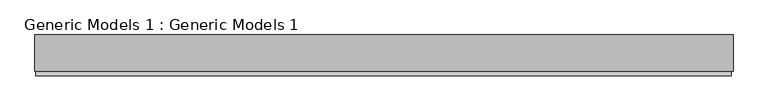
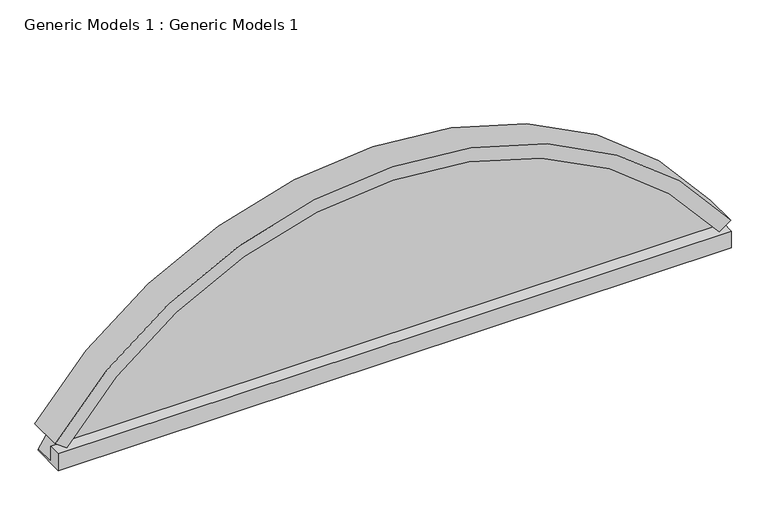
"""IFC4 building model written with IfcOpenShell, lengths in millimetres: proxy geometry, Generic Models 1 : Generic Models 1."""

from ifc_helpers import new_model, si_unit, point, frame, frame_2d, origin, place, context, project, spatial, polyline, circle_curve, trimmed, segment, composite_curve, outline, extrude, source, transform, mapped, element, save
from ifc_brep_helpers import plane_surface, cylinder_surface, revolved_surface, advanced_brep


def generic_models_1_generic_models_1_1dae4af3(model_context):
    return source(origin(), model_context, "Body", "SolidModel", [
        advanced_brep(
        [(-14032.5422477, 3869.5372166, 2197.1), (-14074.0083114, 3869.5372166, 2226.4463041), (-14074.0083114, 3996.5372166, 2226.4463041), (-14032.5422477, 3996.5372166, 2197.1), (-14032.5422477, 3902.5572166, 2197.1), (-11668.9766173, 3869.5372166, 2197.1), (-11668.9766173, 3902.5572166, 2197.1), (-11668.9766173, 3996.5372166, 2197.1), (-11627.5105536, 3996.5372166, 2226.4463041), (-11627.5105536, 3869.5372166, 2226.4463041)],
        [
            (0, 1),
            (1, 2),
            (2, 3),
            (3, 4),
            (4, 0),
            (5, 6),
            (6, 7),
            (7, 8),
            (8, 9),
            (9, 5),
            (9, 1, circle_curve(frame((-12850.7594325, 3869.5372166, 1360.7303343), z_axis=(0.0, -1.0, 0.0), x_axis=(-0.816261096282117, 0.0, 0.5776831507810458)), 1498.6)),
            (0, 5, circle_curve(frame((-12850.7594325, 3869.5372166, 1360.7303343), z_axis=(0.0, 1.0, 0.0), x_axis=(-0.816261096282117, 0.0, 0.5776831507810458)), 1447.8)),
            (8, 2, circle_curve(frame((-12850.7594325, 3996.5372166, 1360.7303343), z_axis=(0.0, -1.0, 0.0), x_axis=(-0.816261096282117, 0.0, 0.5776831507810458)), 1498.6)),
            (7, 3, circle_curve(frame((-12850.7594325, 3996.5372166, 1360.7303343), z_axis=(0.0, -1.0, 0.0), x_axis=(-0.816261096282117, 0.0, 0.5776831507810458)), 1447.8)),
            (6, 4, circle_curve(frame((-12850.7594325, 3902.5572166, 1360.7303343), z_axis=(0.0, -1.0, 0.0), x_axis=(-0.816261096282117, 0.0, 0.5776831507810458)), 1447.8)),
        ],
        [
            plane_surface(frame((-14032.5422477, 3902.5572166, 2197.1), z_axis=(-0.5776831507810458, 0.0, -0.816261096282117), x_axis=(0.0, -1.0, 0.0))),
            plane_surface(frame((-11668.9766173, 3902.5572166, 2197.1), z_axis=(0.5776831507810668, 0.0, -0.8162610962821022), x_axis=(0.0, -1.0, 0.0))),
            plane_surface(frame((-12850.7594325, 3869.5372166, 1360.7303343), z_axis=(0.0, -1.0, 0.0), x_axis=(-0.816261096282117, 0.0, 0.5776831507810458))),
            cylinder_surface(frame((-12850.7594325, 3902.5572166, 1360.7303343), z_axis=(0.0, 1.0, 0.0), x_axis=(-0.816261096282117, 0.0, 0.5776831507810458)), 1498.6),
            plane_surface(frame((-12850.7594325, 3996.5372166, 1360.7303343), z_axis=(0.0, 1.0, 0.0), x_axis=(-0.816261096282117, 0.0, 0.5776831507810458))),
            revolved_surface(polyline([(-14032.542247697249, 3996.5372166, 2197.100000000798), (-14032.542247697249, 3902.5572166, 2197.100000000798)]), (-12850.7594325, 3902.5572166, 1360.7303343), (0.0, 1.0, 0.0)),
            revolved_surface(polyline([(-14032.542247697249, 3902.5572166, 2197.100000000798), (-14032.542247697249, 3869.5372166, 2197.100000000798)]), (-12850.7594325, 3902.5572166, 1360.7303343), (0.0, 1.0, 0.0)),
        ],
        [
            (0, [[1, 2, 3, 4, 5]]),
            (1, [[6, 7, 8, 9, 10]]),
            (2, [[11, -1, 12, -10]]),
            (3, [[13, -2, -11, -9]]),
            (4, [[14, -3, -13, -8]]),
            (5, [[15, -4, -14, -7]]),
            (6, [[-12, -5, -15, -6]]),
        ],
    ),
        extrude(outline(composite_curve([segment(polyline([(2197.1, -14032.5422477), (2197.1, -11668.9766173)]), True, "CONTINUOUS"), segment(trimmed(circle_curve(frame_2d((1360.7303343, -12850.7594325)), 1447.8), [point((2197.1, -11668.9766173))], [point((2197.1, -14032.5422477))], False, "CARTESIAN"), True, "CONTINUOUS")], self_intersect=False)), frame((0.0, 3902.5572166, 0.0), z_axis=(0.0, 1.0, 0.0), x_axis=(0.0, 0.0, 1.0)), (0.0, 0.0, 1.0), 25.4),
        advanced_brep(
        [(-14071.7736637, 3853.6170165, 2197.1), (-11633.6590017, 3853.6170165, 2197.1), (-11633.6590017, 3902.5572166, 2197.1), (-11668.9766173, 3902.5572166, 2197.1), (-11668.9766173, 3980.6170165, 2197.1), (-14032.5422477, 3980.6170165, 2197.1), (-14032.5422477, 3902.5572166, 2197.1), (-14071.7736637, 3902.5572166, 2197.1), (-11633.6590017, 3980.6170165, 2133.6), (-11633.6590017, 3853.6170165, 2133.6), (-14071.7736637, 3853.6170165, 2133.6), (-14071.7736637, 3980.6170165, 2133.6), (-14071.7736637, 3980.6170165, 2138.7078965), (-11633.6590017, 3980.6170165, 2144.8166696), (-14071.7736637, 3902.5572166, 2138.7078965), (-11633.6590017, 3902.5572166, 2144.8166696)],
        [
            (0, 1),
            (1, 2),
            (2, 3),
            (3, 4),
            (4, 5),
            (5, 6),
            (6, 7),
            (7, 0),
            (8, 9),
            (9, 10),
            (10, 11),
            (11, 8),
            (11, 12),
            (12, 5, circle_curve(frame((-12850.7594325, 3980.6170165, 1360.7303343), z_axis=(0.0, 1.0, 0.0), x_axis=(1.0, 0.0, 0.0)), 1447.8)),
            (4, 13, circle_curve(frame((-12850.7594325, 3980.6170165, 1360.7303343), z_axis=(0.0, 1.0, 0.0), x_axis=(1.0, 0.0, 0.0)), 1447.8)),
            (13, 8),
            (10, 0),
            (7, 14),
            (14, 12),
            (9, 1),
            (13, 15),
            (15, 2),
            (15, 3, circle_curve(frame((-12850.7594325, 3902.5572166, 1360.7303343), z_axis=(0.0, -1.0, 0.0), x_axis=(1.0, 0.0, 0.0)), 1447.8)),
            (6, 14, circle_curve(frame((-12850.7594325, 3902.5572166, 1360.7303343), z_axis=(0.0, -1.0, 0.0), x_axis=(1.0, 0.0, 0.0)), 1447.8)),
        ],
        [
            plane_surface(frame((-14071.7736637, 3980.6170165, 2197.1), z_axis=(0.0, 0.0, 1.0), x_axis=(-1.0, 0.0, 0.0))),
            plane_surface(frame((-14071.7736637, 3980.6170165, 2133.6), z_axis=(0.0, 0.0, -1.0), x_axis=(1.0, 0.0, 0.0))),
            plane_surface(frame((-11633.6590017, 3980.6170165, 2197.1), z_axis=(0.0, 1.0, 0.0), x_axis=(0.0, 0.0, -1.0))),
            plane_surface(frame((-14071.7736637, 3980.6170165, 2197.1), z_axis=(-1.0, 0.0, 0.0), x_axis=(0.0, 0.0, -1.0))),
            plane_surface(frame((-14071.7736637, 3853.6170165, 2197.1), z_axis=(0.0, -1.0, 0.0), x_axis=(0.0, 0.0, -1.0))),
            plane_surface(frame((-11633.6590017, 3853.6170165, 2197.1), z_axis=(1.0, 0.0, 0.0), x_axis=(0.0, 0.0, -1.0))),
            plane_surface(frame((-11402.9594325, 3902.5572166, 1360.7303343), z_axis=(0.0, 1.0, 0.0), x_axis=(0.0, 0.0, -1.0))),
            cylinder_surface(frame((-12850.7594325, 3902.5572166, 1360.7303343), z_axis=(0.0, -1.0, 0.0), x_axis=(1.0, 0.0, 0.0)), 1447.8),
        ],
        [
            (0, [[1, 2, 3, 4, 5, 6, 7, 8]]),
            (1, [[9, 10, 11, 12]]),
            (2, [[-12, 13, 14, -5, 15, 16]]),
            (3, [[-11, 17, -8, 18, 19, -13]]),
            (4, [[-1, -17, -10, 20]]),
            (5, [[-9, -16, 21, 22, -2, -20]]),
            (6, [[23, -3, -22]]),
            (6, [[24, -18, -7]]),
            (7, [[-23, -21, -15, -4]]),
            (7, [[-24, -6, -14, -19]]),
        ],
    ),
    ])


if __name__ == "__main__":
    model = new_model("IFC4")
    model_context = context("Model", 3, world=origin())
    ifc_project = project(units=[si_unit("LENGTHUNIT", "METRE", prefix="MILLI")], contexts=[model_context])
    site = spatial("IfcSite", under=ifc_project)
    building = spatial("IfcBuilding", under=site)
    placement = place(None, origin())
    generic_models_1_generic_models_1_shape = generic_models_1_generic_models_1_1dae4af3(model_context)
    element("IfcBuildingElementProxy", 1, Name="Generic Models 1 : Generic Models 1", ObjectType="Generic Models 1 : Generic Models 1", at=placement, inside=building, context=model_context, shape_type="MappedRepresentation", body=[
        mapped(generic_models_1_generic_models_1_shape, transform((0.0, 0.0, 0.0), x_axis=(1.0, 0.0, 0.0), y_axis=(0.0, 1.0, 0.0), z_axis=(0.0, 0.0, 1.0))),
    ])
    save(model, "model.ifc")

# Revit data of these elements
# Element 1 (IfcBuildingElementProxy, "Generic Models 1 : Generic Models 1")
#   Materials on its faces: "Gypsum Wall Board", "Glass"
# Materials
#   "Gypsum Wall Board": class "Generic", colour RGB 228 228 228, transparency 0, Description = "Gypsum Wall Board", Cost = 0
#   "Glass": class "Glass", colour RGB 154 182 205, transparency 0.85, Description = "Soda Lime Glass", Cost = 0
